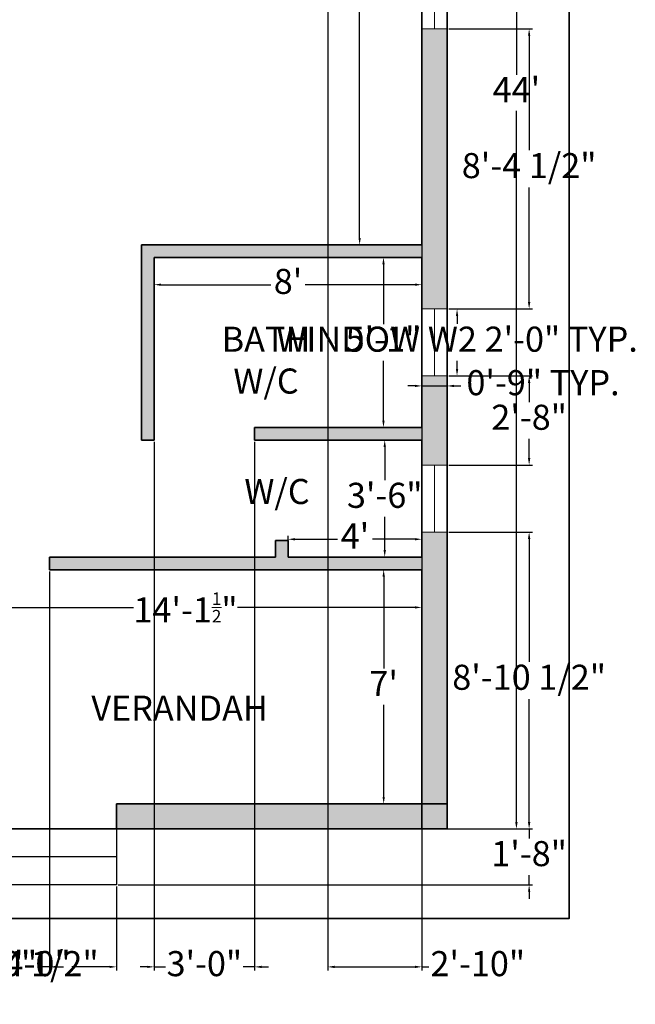
# Model space of a CAD drawing. Units: inches. Extents: x 4987 to 5457, y 8145 to 8785.
# Tile 2 of 3: x 5237 to 5457, y 8145 to 8498. Entities that reach past the tile are written whole.
import ezdxf

# ---------------------------------------------------------------- set-up
doc = ezdxf.new("R2010")
doc.units = ezdxf.units.IN
for name, color, linetype, lineweight in [('A-ANNO-DIMS', 2, 'Continuous', 18), ('A-ANNO-TTLB', 7, 'Continuous', 35), ('A-AREA-IDEN', 240, 'Continuous', 25), ('A-COLS', 7, 'Continuous', 35), ('A-COLS-PATT', 7, 'Continuous', 13), ('A-FLOR-STRS', 7, 'Continuous', 25), ('A-GLAZ', 4, 'Continuous', 18), ('A-WALL', 7, 'Continuous', 35)]:
    doc.layers.add(name, color=color, linetype=linetype, lineweight=lineweight)
doc.layers.add('A-WALL-PATT', color=67, linetype='Continuous', lineweight=13, true_color=0x727430)
doc.styles.get("Standard").update_dxf_attribs({"font": 'arial.ttf'})
doc.dimstyles.new('ISO-25', dxfattribs={"dimtxt": 9, "dimasz": 2.5, "dimexe": 1.25, "dimexo": 0.625, "dimgap": 2, "dimtad": 0, "dimtih": 1, "dimtoh": 1, "dimdec": 1, "dimlunit": 4, "dimtxsty": 'Standard', "dimcen": 2.5, "dimadec": 0, "dimazin": 0, "dimtfac": 0.5, "dimtdec": 1, "dimtmove": 0, "dimatfit": 3, "dimfxl": 1, "dimarcsym": 0})

# ---------------------------------------------------------------- blocks, each defined once
blk = doc.blocks.new('*D3')
at = {"layer": 'A-ANNO-DIMS', "color": 0, "lineweight": -2, "transparency": 16777216}
for p, q in [((5380.22, 8620.24), (5357.27, 8620.24)), ((5358.52, 8617.74), (5358.52, 8525.33)), ((5358.52, 8419.74), (5358.52, 8512.14)), ((5380.22, 8417.24), (5357.27, 8417.24))]:
    blk.add_line(p, q, dxfattribs=at)
at = {"layer": 'A-ANNO-DIMS', "color": 0, "transparency": 16777216}
for points in [[(5358.11, 8617.74), (5358.94, 8617.74), (5358.52, 8620.24)], [(5358.11, 8419.74), (5358.94, 8419.74), (5358.52, 8417.24)]]:
    blk.add_solid(points, dxfattribs=at)
at = {"layer": 'Defpoints', "color": 0, "transparency": 16777216}
for p in [(5380.84, 8620.24), (5358.52, 8417.24), (5380.84, 8417.24)]:
    blk.add_point(p, dxfattribs=at)
at = {"layer": 'A-ANNO-DIMS', "color": 0, "transparency": 16777216, "insert": (5358.52, 8518.74), "char_height": 9, "attachment_point": 5}
blk.add_mtext('16\'-11"', dxfattribs=at)
blk = doc.blocks.new('*D11')
at = {"layer": 'A-ANNO-DIMS', "color": 0, "lineweight": -2, "transparency": 16777216}
for p, q in [((5284.84, 8412.11), (5284.84, 8401.7)), ((5380.84, 8412.11), (5380.84, 8401.7)), ((5287.34, 8402.95), (5326.69, 8402.95)), ((5378.34, 8402.95), (5338.99, 8402.95))]:
    blk.add_line(p, q, dxfattribs=at)
at = {"layer": 'A-ANNO-DIMS', "color": 0, "transparency": 16777216}
for points in [[(5287.34, 8403.37), (5287.34, 8402.54), (5284.84, 8402.95)], [(5378.34, 8403.37), (5378.34, 8402.54), (5380.84, 8402.95)]]:
    blk.add_solid(points, dxfattribs=at)
at = {"layer": 'Defpoints', "color": 0, "transparency": 16777216}
for p in [(5284.84, 8412.74), (5380.84, 8412.74), (5380.84, 8402.95)]:
    blk.add_point(p, dxfattribs=at)
at = {"layer": 'A-ANNO-DIMS', "color": 0, "transparency": 16777216, "insert": (5332.84, 8402.95), "char_height": 9, "attachment_point": 5}
blk.add_mtext("8'", dxfattribs=at)
blk = doc.blocks.new('*D12')
at = {"layer": 'A-ANNO-DIMS', "color": 0, "lineweight": -2, "transparency": 16777216}
for p, q in [((5380.22, 8412.74), (5365.82, 8412.74)), ((5367.07, 8410.24), (5367.07, 8388.83)), ((5367.07, 8354.24), (5367.07, 8375.64)), ((5380.22, 8351.74), (5365.82, 8351.74))]:
    blk.add_line(p, q, dxfattribs=at)
at = {"layer": 'A-ANNO-DIMS', "color": 0, "transparency": 16777216}
for points in [[(5366.65, 8410.24), (5367.49, 8410.24), (5367.07, 8412.74)], [(5366.65, 8354.24), (5367.49, 8354.24), (5367.07, 8351.74)]]:
    blk.add_solid(points, dxfattribs=at)
at = {"layer": 'Defpoints', "color": 0, "transparency": 16777216}
for p in [(5367.07, 8412.74), (5380.84, 8412.74), (5380.84, 8351.74)]:
    blk.add_point(p, dxfattribs=at)
at = {"layer": 'A-ANNO-DIMS', "color": 0, "transparency": 16777216, "insert": (5367.07, 8382.24), "char_height": 9, "attachment_point": 5}
blk.add_mtext('5\'-1"', dxfattribs=at)
blk = doc.blocks.new('*D13')
at = {"layer": 'A-ANNO-DIMS', "color": 0, "lineweight": -2, "transparency": 16777216}
for p, q in [((5380.22, 8347.24), (5366.26, 8347.24)), ((5367.51, 8344.74), (5367.51, 8332.83)), ((5367.51, 8307.74), (5367.51, 8319.64)), ((5380.22, 8305.24), (5366.26, 8305.24))]:
    blk.add_line(p, q, dxfattribs=at)
at = {"layer": 'A-ANNO-DIMS', "color": 0, "transparency": 16777216}
for points in [[(5367.1, 8344.74), (5367.93, 8344.74), (5367.51, 8347.24)], [(5367.1, 8307.74), (5367.93, 8307.74), (5367.51, 8305.24)]]:
    blk.add_solid(points, dxfattribs=at)
at = {"layer": 'Defpoints', "color": 0, "transparency": 16777216}
for p in [(5380.84, 8347.24), (5367.51, 8305.24), (5380.84, 8305.24)]:
    blk.add_point(p, dxfattribs=at)
at = {"layer": 'A-ANNO-DIMS', "color": 0, "transparency": 16777216, "insert": (5367.51, 8326.24), "char_height": 9, "attachment_point": 5}
blk.add_mtext('3\'-6"', dxfattribs=at)
blk = doc.blocks.new('*D14')
at = {"layer": 'A-ANNO-DIMS', "color": 0, "lineweight": -2, "transparency": 16777216}
for p, q in [((5332.84, 8305.86), (5332.84, 8312.9)), ((5380.84, 8305.86), (5380.84, 8312.9)), ((5335.34, 8311.65), (5350.52, 8311.65)), ((5378.34, 8311.65), (5363.16, 8311.65))]:
    blk.add_line(p, q, dxfattribs=at)
at = {"layer": 'A-ANNO-DIMS', "color": 0, "transparency": 16777216}
for points in [[(5335.34, 8312.06), (5335.34, 8311.23), (5332.84, 8311.65)], [(5378.34, 8312.06), (5378.34, 8311.23), (5380.84, 8311.65)]]:
    blk.add_solid(points, dxfattribs=at)
at = {"layer": 'Defpoints', "color": 0, "transparency": 16777216}
for p in [(5380.84, 8311.65), (5332.84, 8305.24), (5380.84, 8305.24)]:
    blk.add_point(p, dxfattribs=at)
at = {"layer": 'A-ANNO-DIMS', "color": 0, "transparency": 16777216, "insert": (5356.84, 8311.65), "char_height": 9, "attachment_point": 5}
blk.add_mtext("4'", dxfattribs=at)
blk = doc.blocks.new('*D15')
at = {"layer": 'A-ANNO-DIMS', "color": 0, "lineweight": -2, "transparency": 16777216}
for p, q in [((5380.22, 8300.74), (5365.89, 8300.74)), ((5367.14, 8298.24), (5367.14, 8265.24)), ((5367.14, 8219.24), (5367.14, 8252.24)), ((5380.22, 8216.74), (5365.89, 8216.74))]:
    blk.add_line(p, q, dxfattribs=at)
at = {"layer": 'A-ANNO-DIMS', "color": 0, "transparency": 16777216}
for points in [[(5366.72, 8298.24), (5367.56, 8298.24), (5367.14, 8300.74)], [(5366.72, 8219.24), (5367.56, 8219.24), (5367.14, 8216.74)]]:
    blk.add_solid(points, dxfattribs=at)
at = {"layer": 'Defpoints', "color": 0, "transparency": 16777216}
for p in [(5367.14, 8300.74), (5380.84, 8300.74), (5380.84, 8216.74)]:
    blk.add_point(p, dxfattribs=at)
at = {"layer": 'A-ANNO-DIMS', "color": 0, "transparency": 16777216, "insert": (5367.14, 8258.74), "char_height": 9, "attachment_point": 5}
blk.add_mtext("7'", dxfattribs=at)
blk = doc.blocks.new('*D16')
at = {"layer": 'A-ANNO-DIMS', "color": 0, "lineweight": -2, "transparency": 16777216}
for p, q in [((5211.34, 8300.11), (5211.34, 8285.95)), ((5380.84, 8300.11), (5380.84, 8285.95)), ((5213.84, 8287.2), (5277.41, 8287.2)), ((5378.34, 8287.2), (5314.77, 8287.2))]:
    blk.add_line(p, q, dxfattribs=at)
at = {"layer": 'A-ANNO-DIMS', "color": 0, "transparency": 16777216}
for points in [[(5213.84, 8287.62), (5213.84, 8286.79), (5211.34, 8287.2)], [(5378.34, 8287.62), (5378.34, 8286.79), (5380.84, 8287.2)]]:
    blk.add_solid(points, dxfattribs=at)
at = {"layer": 'Defpoints', "color": 0, "transparency": 16777216}
for p in [(5211.34, 8300.74), (5380.84, 8300.74), (5211.34, 8287.2)]:
    blk.add_point(p, dxfattribs=at)
at = {"layer": 'A-ANNO-DIMS', "color": 0, "transparency": 16777216, "insert": (5296.09, 8287.2), "char_height": 9, "attachment_point": 5}
blk.add_mtext('14\'-1{\\H0.5x;\\S1/2;}"', dxfattribs=at)
blk = doc.blocks.new('*D19')
at = {"layer": 'A-ANNO-DIMS', "color": 0, "lineweight": -2, "transparency": 16777216}
for p, q in [((5390.47, 8735.74), (5415.98, 8735.74)), ((5414.73, 8733.24), (5414.73, 8478.24)), ((5414.73, 8210.24), (5414.73, 8465.24)), ((5390.47, 8207.74), (5415.98, 8207.74))]:
    blk.add_line(p, q, dxfattribs=at)
at = {"layer": 'A-ANNO-DIMS', "color": 0, "transparency": 16777216}
for points in [[(5414.31, 8733.24), (5415.15, 8733.24), (5414.73, 8735.74)], [(5414.31, 8210.24), (5415.15, 8210.24), (5414.73, 8207.74)]]:
    blk.add_solid(points, dxfattribs=at)
at = {"layer": 'Defpoints', "color": 0, "transparency": 16777216}
for p in [(5389.84, 8735.74), (5389.84, 8207.74), (5414.73, 8207.74)]:
    blk.add_point(p, dxfattribs=at)
at = {"layer": 'A-ANNO-DIMS', "color": 0, "transparency": 16777216, "insert": (5414.73, 8471.74), "char_height": 9, "attachment_point": 5}
blk.add_mtext("44'", dxfattribs=at)
blk = doc.blocks.new('WIN-48IN')
for p, q in [((0, 0), (0, 9)), ((48, 0), (48, 9)), ((0, 4.5), (48, 4.5))]:
    blk.add_line(p, q)
blk = doc.blocks.new('WIN-24IN')
for p, q in [((0, 24), (9, 24)), ((4.5, 24), (4.5, 0)), ((0, 0), (9, 0))]:
    blk.add_line(p, q)
blk = doc.blocks.new('COL-CORNER-9IN')
for q in [(0, 0), (9, 9)]:
    blk.add_line((0, 9), q)
blk = doc.blocks.new('*D26')
at = {"layer": 'A-ANNO-DIMS', "color": 0, "lineweight": -2, "transparency": 16777216}
for p, q in [((5390.47, 8394.24), (5394.69, 8394.24)), ((5393.44, 8391.74), (5393.44, 8388.89)), ((5393.44, 8372.74), (5393.44, 8375.58)), ((5390.47, 8370.24), (5394.69, 8370.24))]:
    blk.add_line(p, q, dxfattribs=at)
at = {"layer": 'A-ANNO-DIMS', "color": 0, "transparency": 16777216}
for points in [[(5393.02, 8391.74), (5393.86, 8391.74), (5393.44, 8394.24)], [(5393.02, 8372.74), (5393.86, 8372.74), (5393.44, 8370.24)]]:
    blk.add_solid(points, dxfattribs=at)
at = {"layer": 'Defpoints', "color": 0, "transparency": 16777216}
for p in [(5389.84, 8394.24), (5393.44, 8394.24), (5389.84, 8370.24)]:
    blk.add_point(p, dxfattribs=at)
at = {"layer": 'A-ANNO-DIMS', "color": 0, "transparency": 16777216, "insert": (5393.44, 8382.24), "char_height": 9, "attachment_point": 5}
blk.add_mtext('WINDOW W2 2\'-0" TYP.', dxfattribs=at)
blk = doc.blocks.new('*D27')
at = {"layer": 'A-ANNO-DIMS', "color": 0, "lineweight": -2, "transparency": 16777216}
for p, q in [((5380.84, 8369.61), (5380.84, 8365.39)), ((5389.84, 8369.61), (5389.84, 8365.39)), ((5378.34, 8366.64), (5375.84, 8366.64)), ((5380.84, 8366.64), (5389.84, 8366.64)), ((5392.34, 8366.64), (5394.84, 8366.64))]:
    blk.add_line(p, q, dxfattribs=at)
at = {"layer": 'A-ANNO-DIMS', "color": 0, "transparency": 16777216}
for points in [[(5378.34, 8367.05), (5378.34, 8366.22), (5380.84, 8366.64)], [(5392.34, 8367.05), (5392.34, 8366.22), (5389.84, 8366.64)]]:
    blk.add_solid(points, dxfattribs=at)
at = {"layer": 'Defpoints', "color": 0, "transparency": 16777216}
for p in [(5380.84, 8370.24), (5389.84, 8370.24), (5389.84, 8366.64)]:
    blk.add_point(p, dxfattribs=at)
at = {"layer": 'A-ANNO-DIMS', "color": 0, "transparency": 16777216, "insert": (5424.27, 8366.64), "char_height": 9, "attachment_point": 5}
blk.add_mtext('0\'-9" TYP.', dxfattribs=at)
blk = doc.blocks.new('*D33')
at = {"layer": 'A-ANNO-DIMS', "color": 0, "lineweight": -2, "transparency": 16777216}
for p, q in [((5390.47, 8314.24), (5420.54, 8314.24)), ((5419.29, 8311.74), (5419.29, 8267.64)), ((5419.29, 8210.24), (5419.29, 8254.33)), ((5390.47, 8207.74), (5420.54, 8207.74))]:
    blk.add_line(p, q, dxfattribs=at)
at = {"layer": 'A-ANNO-DIMS', "color": 0, "transparency": 16777216}
for points in [[(5418.87, 8311.74), (5419.71, 8311.74), (5419.29, 8314.24)], [(5418.87, 8210.24), (5419.71, 8210.24), (5419.29, 8207.74)]]:
    blk.add_solid(points, dxfattribs=at)
at = {"layer": 'Defpoints', "color": 0, "transparency": 16777216}
for p in [(5389.84, 8314.24), (5419.29, 8314.24), (5389.84, 8207.74)]:
    blk.add_point(p, dxfattribs=at)
at = {"layer": 'A-ANNO-DIMS', "color": 0, "transparency": 16777216, "insert": (5419.29, 8260.99), "char_height": 9, "attachment_point": 5}
blk.add_mtext('8\'-10 1/2"', dxfattribs=at)
blk = doc.blocks.new('*D34')
at = {"layer": 'A-ANNO-DIMS', "color": 0, "lineweight": -2, "transparency": 16777216}
for p, q in [((5390.47, 8370.24), (5420.54, 8370.24)), ((5419.29, 8367.74), (5419.29, 8360.83)), ((5419.29, 8340.74), (5419.29, 8347.64)), ((5390.47, 8338.24), (5420.54, 8338.24))]:
    blk.add_line(p, q, dxfattribs=at)
at = {"layer": 'A-ANNO-DIMS', "color": 0, "transparency": 16777216}
for points in [[(5418.87, 8367.74), (5419.71, 8367.74), (5419.29, 8370.24)], [(5418.87, 8340.74), (5419.71, 8340.74), (5419.29, 8338.24)]]:
    blk.add_solid(points, dxfattribs=at)
at = {"layer": 'Defpoints', "color": 0, "transparency": 16777216}
for p in [(5389.84, 8370.24), (5419.29, 8370.24), (5389.84, 8338.24)]:
    blk.add_point(p, dxfattribs=at)
at = {"layer": 'A-ANNO-DIMS', "color": 0, "transparency": 16777216, "insert": (5419.29, 8354.24), "char_height": 9, "attachment_point": 5}
blk.add_mtext('2\'-8"', dxfattribs=at)
blk = doc.blocks.new('*D35')
at = {"layer": 'A-ANNO-DIMS', "color": 0, "lineweight": -2, "transparency": 16777216}
for p, q in [((5390.47, 8494.74), (5420.54, 8494.74)), ((5419.29, 8492.24), (5419.29, 8451.14)), ((5419.29, 8396.74), (5419.29, 8437.83)), ((5390.47, 8394.24), (5420.54, 8394.24))]:
    blk.add_line(p, q, dxfattribs=at)
at = {"layer": 'A-ANNO-DIMS', "color": 0, "transparency": 16777216}
for points in [[(5418.87, 8492.24), (5419.71, 8492.24), (5419.29, 8494.74)], [(5418.87, 8396.74), (5419.71, 8396.74), (5419.29, 8394.24)]]:
    blk.add_solid(points, dxfattribs=at)
at = {"layer": 'Defpoints', "color": 0, "transparency": 16777216}
for p in [(5389.84, 8494.74), (5419.29, 8494.74), (5389.84, 8394.24)]:
    blk.add_point(p, dxfattribs=at)
at = {"layer": 'A-ANNO-DIMS', "color": 0, "transparency": 16777216, "insert": (5419.29, 8444.49), "char_height": 9, "attachment_point": 5}
blk.add_mtext('8\'-4 1/2"', dxfattribs=at)
blk = doc.blocks.new('*D37')
at = {"layer": 'A-ANNO-DIMS', "color": 0, "lineweight": -2, "transparency": 16777216}
for p, q in [((5211.34, 8187.11), (5211.34, 8157.04)), ((5271.34, 8187.11), (5271.34, 8157.04)), ((5213.84, 8158.29), (5227.38, 8158.29)), ((5268.84, 8158.29), (5255.3, 8158.29))]:
    blk.add_line(p, q, dxfattribs=at)
at = {"layer": 'A-ANNO-DIMS', "color": 0, "transparency": 16777216}
for points in [[(5213.84, 8158.7), (5213.84, 8157.87), (5211.34, 8158.29)], [(5268.84, 8158.7), (5268.84, 8157.87), (5271.34, 8158.29)]]:
    blk.add_solid(points, dxfattribs=at)
at = {"layer": 'Defpoints', "color": 0, "transparency": 16777216}
for p in [(5211.34, 8187.74), (5271.34, 8187.74), (5271.34, 8158.29)]:
    blk.add_point(p, dxfattribs=at)
at = {"layer": 'A-ANNO-DIMS', "color": 0, "transparency": 16777216, "insert": (5241.34, 8158.29), "char_height": 9, "attachment_point": 5}
blk.add_mtext('5\'-0"', dxfattribs=at)
blk = doc.blocks.new('*D38')
at = {"layer": 'A-ANNO-DIMS', "color": 0, "lineweight": -2, "transparency": 16777216}
for p, q in [((5419.29, 8210.24), (5419.29, 8212.74)), ((5271.97, 8207.74), (5420.54, 8207.74)), ((5419.29, 8207.74), (5419.29, 8204.33)), ((5419.29, 8187.74), (5419.29, 8191.14)), ((5271.97, 8187.74), (5420.54, 8187.74)), ((5419.29, 8185.24), (5419.29, 8182.74))]:
    blk.add_line(p, q, dxfattribs=at)
at = {"layer": 'A-ANNO-DIMS', "color": 0, "transparency": 16777216}
for points in [[(5418.87, 8210.24), (5419.71, 8210.24), (5419.29, 8207.74)], [(5418.87, 8185.24), (5419.71, 8185.24), (5419.29, 8187.74)]]:
    blk.add_solid(points, dxfattribs=at)
at = {"layer": 'Defpoints', "color": 0, "transparency": 16777216}
for p in [(5271.34, 8207.74), (5419.29, 8207.74), (5271.34, 8187.74)]:
    blk.add_point(p, dxfattribs=at)
at = {"layer": 'A-ANNO-DIMS', "color": 0, "transparency": 16777216, "insert": (5419.29, 8197.74), "char_height": 9, "attachment_point": 5}
blk.add_mtext('1\'-8"', dxfattribs=at)
blk = doc.blocks.new('*D42')
at = {"layer": 'A-ANNO-DIMS', "color": 0, "lineweight": -2, "transparency": 16777216}
for p, q in [((5347.07, 8624.11), (5347.07, 8157.04)), ((5380.84, 8624.11), (5380.84, 8157.04)), ((5349.57, 8158.29), (5378.34, 8158.29)), ((5380.84, 8158.29), (5383.34, 8158.29))]:
    blk.add_line(p, q, dxfattribs=at)
at = {"layer": 'A-ANNO-DIMS', "color": 0, "transparency": 16777216}
for points in [[(5349.57, 8158.7), (5349.57, 8157.87), (5347.07, 8158.29)], [(5378.34, 8158.7), (5378.34, 8157.87), (5380.84, 8158.29)]]:
    blk.add_solid(points, dxfattribs=at)
at = {"layer": 'Defpoints', "color": 0, "transparency": 16777216}
for p in [(5347.07, 8624.74), (5380.84, 8624.74), (5380.84, 8158.29)]:
    blk.add_point(p, dxfattribs=at)
at = {"layer": 'A-ANNO-DIMS', "color": 0, "transparency": 16777216, "insert": (5400.88, 8158.29), "char_height": 9, "attachment_point": 5}
blk.add_mtext('2\'-10"', dxfattribs=at)
blk = doc.blocks.new('*D48')
at = {"layer": 'A-ANNO-DIMS', "color": 0, "lineweight": -2, "transparency": 16777216}
for p, q in [((5284.84, 8346.61), (5284.84, 8157.04)), ((5320.84, 8346.61), (5320.84, 8157.04)), ((5282.34, 8158.29), (5279.84, 8158.29)), ((5284.84, 8158.29), (5288.88, 8158.29)), ((5320.84, 8158.29), (5316.8, 8158.29)), ((5323.34, 8158.29), (5325.84, 8158.29))]:
    blk.add_line(p, q, dxfattribs=at)
at = {"layer": 'A-ANNO-DIMS', "color": 0, "transparency": 16777216}
for points in [[(5282.34, 8158.7), (5282.34, 8157.87), (5284.84, 8158.29)], [(5323.34, 8158.7), (5323.34, 8157.87), (5320.84, 8158.29)]]:
    blk.add_solid(points, dxfattribs=at)
at = {"layer": 'Defpoints', "color": 0, "transparency": 16777216}
for p in [(5284.84, 8347.24), (5320.84, 8347.24), (5320.84, 8158.29)]:
    blk.add_point(p, dxfattribs=at)
at = {"layer": 'A-ANNO-DIMS', "color": 0, "transparency": 16777216, "insert": (5302.84, 8158.29), "char_height": 9, "attachment_point": 5}
blk.add_mtext('3\'-0"', dxfattribs=at)
blk = doc.blocks.new('*D49')
at = {"layer": 'A-ANNO-DIMS', "color": 0, "lineweight": -2, "transparency": 16777216}
for p, q in [((5211.34, 8300.11), (5211.34, 8157.04)), ((5247.34, 8300.11), (5247.34, 8157.04)), ((5208.84, 8158.29), (5206.34, 8158.29)), ((5211.34, 8158.29), (5215.38, 8158.29)), ((5247.34, 8158.29), (5243.3, 8158.29)), ((5249.84, 8158.29), (5252.34, 8158.29))]:
    blk.add_line(p, q, dxfattribs=at)
at = {"layer": 'A-ANNO-DIMS', "color": 0, "transparency": 16777216}
for points in [[(5208.84, 8158.7), (5208.84, 8157.87), (5211.34, 8158.29)], [(5249.84, 8158.7), (5249.84, 8157.87), (5247.34, 8158.29)]]:
    blk.add_solid(points, dxfattribs=at)
at = {"layer": 'Defpoints', "color": 0, "transparency": 16777216}
for p in [(5211.34, 8300.74), (5247.34, 8300.74), (5247.34, 8158.29)]:
    blk.add_point(p, dxfattribs=at)
at = {"layer": 'A-ANNO-DIMS', "color": 0, "transparency": 16777216, "insert": (5229.34, 8158.29), "char_height": 9, "attachment_point": 5}
blk.add_mtext('3\'-0"', dxfattribs=at)
blk = doc.blocks.new('*D52')
at = {"layer": 'A-ANNO-DIMS', "color": 0, "lineweight": -2, "transparency": 16777216}
for p, q in [((5206.84, 8252.11), (5206.84, 8157.04)), ((5211.34, 8252.11), (5211.34, 8157.04)), ((5204.34, 8158.29), (5201.84, 8158.29)), ((5206.84, 8158.29), (5211.34, 8158.29)), ((5213.84, 8158.29), (5216.34, 8158.29))]:
    blk.add_line(p, q, dxfattribs=at)
at = {"layer": 'A-ANNO-DIMS', "color": 0, "transparency": 16777216}
for points in [[(5204.34, 8158.7), (5204.34, 8157.87), (5206.84, 8158.29)], [(5213.84, 8158.7), (5213.84, 8157.87), (5211.34, 8158.29)]]:
    blk.add_solid(points, dxfattribs=at)
at = {"layer": 'Defpoints', "color": 0, "transparency": 16777216}
for p in [(5206.84, 8252.74), (5211.34, 8252.74), (5211.34, 8158.29)]:
    blk.add_point(p, dxfattribs=at)
at = {"layer": 'A-ANNO-DIMS', "color": 0, "transparency": 16777216, "insert": (5240.79, 8158.29), "char_height": 9, "attachment_point": 5}
blk.add_mtext('0\'-4 1/2"', dxfattribs=at)

msp = doc.modelspace()

# ---------------------------------------------------------------- hatches: boundary and pattern name
at = {"layer": 'A-COLS-PATT'}
h = msp.add_hatch(color=256, dxfattribs=at)
h.dxf.hatch_style = 1
h.paths.add_polyline_path([(5062.84, 8735.74), (5053.84, 8735.74), (5053.84, 8726.74), (5062.84, 8726.74)])
h.paths.add_polyline_path([(5389.84, 8735.74), (5380.84, 8735.74), (5380.84, 8726.74), (5389.84, 8726.74)])
h.paths.add_polyline_path([(5389.84, 8216.74), (5380.84, 8216.74), (5380.84, 8207.74), (5389.84, 8207.74)])
h.paths.add_polyline_path([(5062.84, 8216.74), (5053.84, 8216.74), (5053.84, 8207.74), (5062.84, 8207.74)])
at = {"layer": 'A-WALL-PATT'}
h = msp.add_hatch(color=256, dxfattribs=at)
h.dxf.hatch_style = 1
h.paths.add_polyline_path([(5220.34, 8735.74), (5062.84, 8735.74), (5062.84, 8726.74), (5111.84, 8726.74), (5220.34, 8726.74)])
h.paths.add_polyline_path([(5062.84, 8548.24), (5053.84, 8548.24), (5053.84, 8453.24), (5062.84, 8453.24), (5062.84, 8495.74), (5206.84, 8495.74), (5211.34, 8495.74), (5211.34, 8500.24), (5206.84, 8500.24), (5062.84, 8500.24)])
h.paths.add_polyline_path([(5211.34, 8362.74), (5211.34, 8412.74), (5211.34, 8417.24), (5211.34, 8459.74), (5206.84, 8459.74), (5206.84, 8417.24), (5206.84, 8412.74), (5206.84, 8362.74), (5062.84, 8362.74), (5062.84, 8405.24), (5053.84, 8405.24), (5053.84, 8311.49), (5062.84, 8311.49), (5062.84, 8358.24), (5206.84, 8358.24), (5211.34, 8358.24)])
h.paths.add_polyline_path([(5062.84, 8263.49), (5053.84, 8263.49), (5053.84, 8216.74), (5062.84, 8216.74)])
h.paths.add_polyline_path([(5211.34, 8216.74), (5206.84, 8216.74), (5062.84, 8216.74), (5062.84, 8207.74), (5211.34, 8207.74)])
h.paths.add_polyline_path([(5380.84, 8216.74), (5271.34, 8216.74), (5271.34, 8207.74), (5380.84, 8207.74)])
h.paths.add_polyline_path([(5389.84, 8314.24), (5380.84, 8314.24), (5380.84, 8305.24), (5332.84, 8305.24), (5332.84, 8311.24), (5328.34, 8311.24), (5328.34, 8305.24), (5247.34, 8305.24), (5247.34, 8300.74), (5380.84, 8300.74), (5380.84, 8216.74), (5389.84, 8216.74)])
h.paths.add_polyline_path([(5389.84, 8370.24), (5380.84, 8370.24), (5380.84, 8351.74), (5328.34, 8351.74), (5320.84, 8351.74), (5320.84, 8347.24), (5328.34, 8347.24), (5332.84, 8347.24), (5380.84, 8347.24), (5380.84, 8338.24), (5389.84, 8338.24)])
h.paths.add_polyline_path([(5389.84, 8494.74), (5380.84, 8494.74), (5380.84, 8417.24), (5280.34, 8417.24), (5280.34, 8412.74), (5280.34, 8351.74), (5280.34, 8347.24), (5284.84, 8347.24), (5284.84, 8351.74), (5284.84, 8412.74), (5328.34, 8412.74), (5380.84, 8412.74), (5380.84, 8394.24), (5389.84, 8394.24)])
h.paths.add_polyline_path([(5389.84, 8726.74), (5380.84, 8726.74), (5380.84, 8624.74), (5272.84, 8624.74), (5268.34, 8624.74), (5268.34, 8620.24), (5380.84, 8620.24), (5380.84, 8542.74), (5389.84, 8542.74)])
h.paths.add_polyline_path([(5062.84, 8726.74), (5053.84, 8726.74), (5053.84, 8596.24), (5062.84, 8596.24), (5062.84, 8644.24), (5062.84, 8648.74)])
h.paths.add_polyline_path([(5302.84, 8735.74), (5268.34, 8735.74), (5268.34, 8726.74), (5268.34, 8660.74), (5272.84, 8660.74), (5272.84, 8726.74), (5302.84, 8726.74)])
h.paths.add_polyline_path([(5380.84, 8735.74), (5350.84, 8735.74), (5350.84, 8726.74), (5380.84, 8726.74)])
h.paths.add_polyline_path([(5211.34, 8648.74), (5206.84, 8648.74), (5098.84, 8648.74), (5098.84, 8644.24), (5206.84, 8644.24), (5206.84, 8624.74), (5206.84, 8536.24), (5211.34, 8536.24), (5211.34, 8620.24), (5211.34, 8624.74)])
h.paths.add_polyline_path([(5211.34, 8305.24), (5211.34, 8322.24), (5206.84, 8322.24), (5206.84, 8305.24), (5206.84, 8300.74), (5206.84, 8252.74), (5211.34, 8252.74), (5211.34, 8300.74)])

# ---------------------------------------------------------------- linework, layer by layer
at = {"layer": 'A-ANNO-TTLB'}
msp.add_lwpolyline([(5031.32, 8785.05), (5433.7, 8785.05), (5433.7, 8175.66), (5031.32, 8175.66)], close=True, dxfattribs=at)
at = {"layer": 'A-FLOR-STRS'}
for p, q in [((5271.34, 8207.74), (5271.34, 8187.74)), ((5271.34, 8197.74), (5211.34, 8197.74)), ((5271.34, 8187.74), (5211.34, 8187.74))]:
    msp.add_line(p, q, dxfattribs=at)
at = {"layer": 'A-WALL'}
for p, q in [((5389.84, 8735.74), (5389.84, 8207.74)), ((5380.84, 8620.24), (5380.84, 8417.24)), ((5284.84, 8417.24), (5280.34, 8417.24)), ((5380.84, 8417.24), (5280.34, 8417.24)), ((5280.34, 8412.74), (5280.34, 8417.24)), ((5284.84, 8417.24), (5328.34, 8417.24)), ((5380.84, 8417.24), (5328.34, 8417.24)), ((5280.34, 8412.74), (5280.34, 8351.74)), ((5284.84, 8412.74), (5284.84, 8351.74)), ((5284.84, 8412.74), (5328.34, 8412.74)), ((5380.84, 8412.74), (5328.34, 8412.74)), ((5380.84, 8412.74), (5380.84, 8351.74)), ((5280.34, 8351.74), (5280.34, 8347.24)), ((5284.84, 8351.74), (5284.84, 8347.24)), ((5320.84, 8351.74), (5328.34, 8351.74)), ((5320.84, 8351.74), (5320.84, 8347.24)), ((5380.84, 8351.74), (5328.34, 8351.74)), ((5284.84, 8347.24), (5280.34, 8347.24)), ((5328.34, 8347.24), (5320.84, 8347.24)), ((5328.34, 8347.24), (5332.84, 8347.24)), ((5380.84, 8347.24), (5332.84, 8347.24)), ((5380.84, 8347.24), (5380.84, 8305.24)), ((5328.34, 8311.24), (5328.34, 8305.24)), ((5328.34, 8311.24), (5332.84, 8311.24)), ((5332.84, 8311.24), (5332.84, 8305.24)), ((5328.34, 8305.24), (5247.34, 8305.24)), ((5247.34, 8305.24), (5247.34, 8300.74)), ((5380.84, 8305.24), (5332.84, 8305.24)), ((5380.84, 8300.74), (5247.34, 8300.74)), ((5380.84, 8300.74), (5380.84, 8216.74)), ((5380.84, 8216.74), (5271.34, 8216.74)), ((5271.34, 8216.74), (5271.34, 8207.74)), ((5389.84, 8207.74), (5053.84, 8207.74))]:
    msp.add_line(p, q, dxfattribs=at)

# ---------------------------------------------------------------- block references
at = {"layer": 'A-COLS'}
msp.add_blockref('COL-CORNER-9IN', (5380.84, 8207.74), dxfattribs=at)
at = {"layer": 'A-GLAZ', "rotation": 90.00000000000134}
msp.add_blockref('WIN-48IN', (5389.84, 8494.73), dxfattribs=at)
at = {"layer": 'A-GLAZ'}
for p in [(5380.84, 8370.24), (5380.84, 8314.24)]:
    msp.add_blockref('WIN-24IN', p, dxfattribs=at)

# ---------------------------------------------------------------- texts
at = {"layer": 'A-AREA-IDEN', "char_height": 9, "attachment_point": 1}
for s, width, insert in [('\\pxqc;{\\fArial|b1|i0|c0|p34;BATH\\PW/C}', 64.3039, (5292.8, 8387.89)), ('\\pxqc;{\\fArial|b1|i0|c0|p34;W/C}', 35.0671, (5311.36, 8333.28)), ('\\pxqc;{\\fArial|b1|i0|c0|p34;VERANDAH}', 103.0969, (5242.41, 8255.56))]:
    msp.add_mtext_dynamic_manual_height_columns(s, width=width, gutter_width=12.5, heights=[0], dxfattribs=dict(at, insert=insert))

# ---------------------------------------------------------------- dimensions: what is measured, and where the dimension line sits
at = {"layer": 'A-ANNO-DIMS'}
for base, p1, p2, override, picture, middle in [((5414.73, 8207.74), (5389.84, 8735.74), (5389.84, 8207.74), {"dimclrd": 0, "dimclre": 0, "dimclrt": 0}, '*D19', (5414.73, 8471.74)), ((5358.52, 8417.24), (5380.84, 8620.24), (5380.84, 8417.24), {"dimclrd": 0, "dimclre": 0, "dimclrt": 0}, '*D3', (5358.52, 8518.74)), ((5419.29, 8494.74), (5389.84, 8394.24), (5389.84, 8494.74), {"dimdec": 1, "dimlfac": 1, "dimrnd": 0, "dimzin": 1, "dimdsep": 46, "dimlunit": 4, "dimfrac": 2}, '*D35', (5419.29, 8444.49)), ((5367.07, 8412.74), (5380.84, 8351.74), (5380.84, 8412.74), {"dimclrd": 0, "dimclre": 0, "dimclrt": 0}, '*D12', (5367.07, 8382.24)), ((5419.29, 8370.24), (5389.84, 8338.24), (5389.84, 8370.24), {"dimdec": 1, "dimlfac": 1, "dimrnd": 0, "dimzin": 1, "dimdsep": 46, "dimlunit": 4, "dimfrac": 2}, '*D34', (5419.29, 8354.24)), ((5367.51, 8305.24), (5380.84, 8347.24), (5380.84, 8305.24), {"dimclrd": 0, "dimclre": 0, "dimclrt": 0}, '*D13', (5367.51, 8326.24)), ((5419.29, 8314.24), (5389.84, 8207.74), (5389.84, 8314.24), {"dimdec": 1, "dimlfac": 1, "dimrnd": 0, "dimzin": 1, "dimdsep": 46, "dimlunit": 4, "dimfrac": 2}, '*D33', (5419.29, 8260.99)), ((5367.14, 8300.74), (5380.84, 8216.74), (5380.84, 8300.74), {"dimclrd": 0, "dimclre": 0, "dimclrt": 0}, '*D15', (5367.14, 8258.74)), ((5419.29, 8207.74), (5271.34, 8187.74), (5271.34, 8207.74), {"dimdec": 1, "dimlfac": 1, "dimrnd": 0, "dimzin": 1, "dimdsep": 46, "dimlunit": 4, "dimfrac": 2}, '*D38', (5419.29, 8197.74))]:
    dim = msp.add_linear_dim(base=base, p1=p1, p2=p2, angle=90, dimstyle='ISO-25', override=override, dxfattribs=at)
    dim.commit()
    dim.dimension.update_dxf_attribs({"geometry": picture, "text_midpoint": middle})
for base, p1, p2, override, picture, middle in [((5380.84, 8158.29), (5347.07, 8624.74), (5380.84, 8624.74), {"dimdec": 1, "dimlfac": 1, "dimrnd": 0, "dimzin": 1, "dimdsep": 46, "dimlunit": 4, "dimfrac": 2}, '*D42', (5400.88, 8158.29)), ((5380.84, 8402.95), (5284.84, 8412.74), (5380.84, 8412.74), {"dimclrd": 0, "dimclre": 0, "dimclrt": 0}, '*D11', (5332.84, 8402.95)), ((5320.84, 8158.29), (5284.84, 8347.24), (5320.84, 8347.24), {"dimdec": 1, "dimlfac": 1, "dimrnd": 0, "dimzin": 1, "dimdsep": 46, "dimlunit": 4, "dimfrac": 2}, '*D48', (5302.84, 8158.29)), ((5380.84, 8311.65), (5332.84, 8305.24), (5380.84, 8305.24), {"dimclrd": 0, "dimclre": 0, "dimclrt": 0}, '*D14', (5356.84, 8311.65)), ((5247.34, 8158.29), (5211.34, 8300.74), (5247.34, 8300.74), {"dimdec": 1, "dimlfac": 1, "dimrnd": 0, "dimzin": 1, "dimdsep": 46, "dimlunit": 4, "dimfrac": 2}, '*D49', (5229.34, 8158.29)), ((5211.34, 8287.2), (5380.84, 8300.74), (5211.34, 8300.74), {"dimclrd": 0, "dimclre": 0, "dimclrt": 0}, '*D16', (5296.09, 8287.2)), ((5211.34, 8158.29), (5206.84, 8252.74), (5211.34, 8252.74), {"dimdec": 1, "dimlfac": 1, "dimrnd": 0, "dimzin": 1, "dimdsep": 46, "dimlunit": 4, "dimfrac": 2}, '*D52', (5240.79, 8158.29)), ((5271.34, 8158.29), (5211.34, 8187.74), (5271.34, 8187.74), {"dimdec": 1, "dimlfac": 1, "dimrnd": 0, "dimzin": 1, "dimdsep": 46, "dimlunit": 4, "dimfrac": 2}, '*D37', (5241.34, 8158.29))]:
    dim = msp.add_linear_dim(base=base, p1=p1, p2=p2, dimstyle='ISO-25', override=override, dxfattribs=at)
    dim.commit()
    dim.dimension.update_dxf_attribs({"geometry": picture, "text_midpoint": middle})
dim = msp.add_linear_dim(base=(5393.44, 8394.24), p1=(5389.84, 8370.24), p2=(5389.84, 8394.24), angle=90, text='WINDOW W2 <> TYP.', dimstyle='ISO-25', override={"dimdec": 1, "dimlfac": 1, "dimrnd": 0, "dimzin": 1, "dimdsep": 46, "dimlunit": 4, "dimfrac": 2}, dxfattribs=at)
dim.commit()
dim.dimension.update_dxf_attribs({"geometry": '*D26', "text_midpoint": (5393.44, 8382.24)})
dim = msp.add_linear_dim(base=(5389.84, 8366.64), p1=(5380.84, 8370.24), p2=(5389.84, 8370.24), text='<> TYP.', dimstyle='ISO-25', override={"dimdec": 1, "dimlfac": 1, "dimrnd": 0, "dimzin": 1, "dimdsep": 46, "dimlunit": 4, "dimfrac": 2}, dxfattribs=at)
dim.commit()
dim.dimension.update_dxf_attribs({"geometry": '*D27', "text_midpoint": (5424.27, 8366.64)})

doc.saveas('drawing.dxf')
